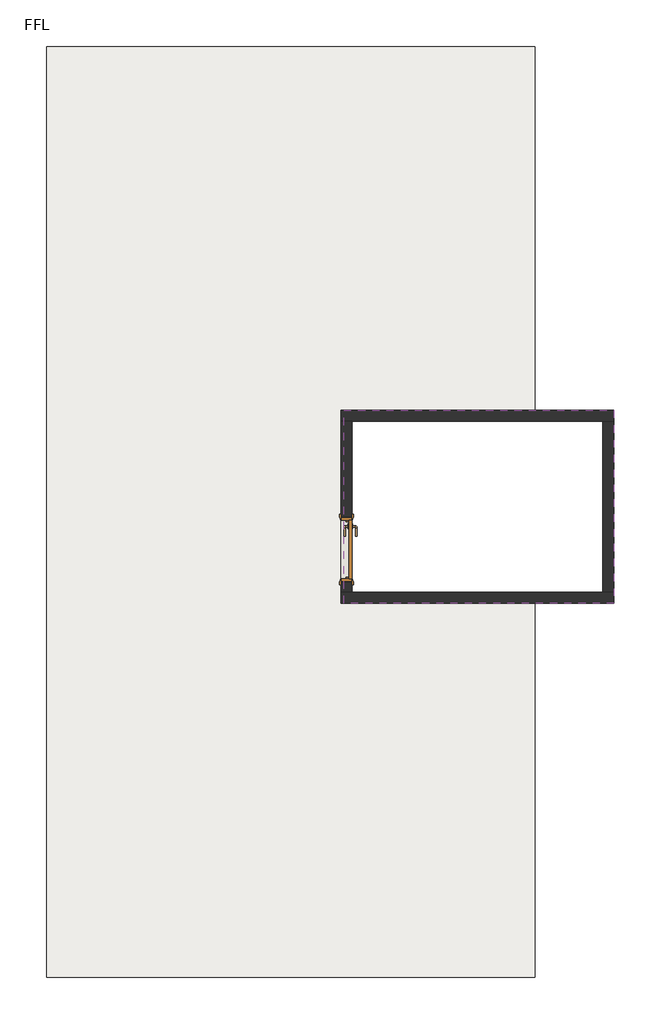
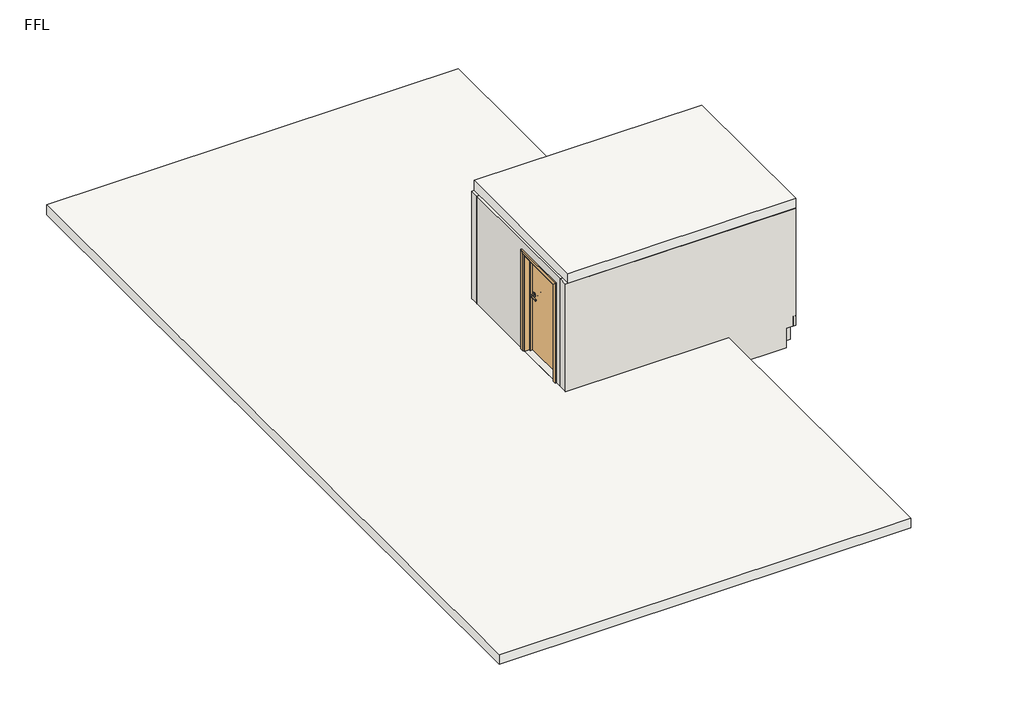
# One storey, incomplete: 4 walls, 3 slabs, 1 door.
"""IFC4 building model written with IfcOpenShell, lengths in millimetres."""

from ifc_helpers import new_model, si_unit, frame, origin, place, context, project, spatial, polyline, outline, extrude, faceted_brep, transform, mapped, element, save
from components import doors_intsgl_810x1524mm_3577b09a

model = new_model("IFC4")

# Units and contexts
model_context = context("Model", 3, world=origin())
ifc_project = project(units=[si_unit("LENGTHUNIT", "METRE", prefix="MILLI")], contexts=[model_context])

# Site, building, storey
site = spatial("IfcSite", under=ifc_project)
building = spatial("IfcBuilding", under=site)
storey = spatial("IfcBuildingStorey", under=building, Name="FFL", Elevation=3048.0)

# Door
placement = place(None, origin())
doors_intsgl_810x1524mm_shape = doors_intsgl_810x1524mm_3577b09a(model_context)
element("IfcDoor", 1, ObjectType="Doors_IntSgl : 810x1524mm", at=placement, inside=storey, context=model_context, shape_type="MappedRepresentation", body=[
    mapped(doors_intsgl_810x1524mm_shape, transform((-2390.6174044, 5851.2803577, 3200.4), x_axis=(0.0, -1.0, 0.0), y_axis=(1.0, 0.0, 0.0), z_axis=(0.0, 0.0, 1.0))),
])

# Slabs
element("IfcSlab", 2, ObjectType="SLAB", at=placement, inside=storey, context=model_context, shape_type="SweptSolid", body=[
    extrude(outline(polyline([(-42.3874044, 12109.5354997), (-42.3874044, 7583.3887671), (-2320.9121226, 7583.3887671), (-2320.9121226, 5180.7203577), (-42.3874044, 5180.7203577), (-42.3874044, 527.1354997), (-6124.4174044, 527.1354997), (-6124.4174044, 12109.5354997), (-42.3874044, 12109.5354997)])), frame((0.0, 0.0, 3048.0), z_axis=(0.0, 0.0, 1.0), x_axis=(1.0, 0.0, 0.0)), (0.0, 0.0, 1.0), 149.9616),
    extrude(outline(polyline([(941.6891182, 7583.3887671), (941.6891182, 5180.7203577), (906.3025956, 5180.7203577), (906.3025956, 7583.3887671), (941.6891182, 7583.3887671)])), frame((0.0, 0.0, 3048.0), z_axis=(0.0, 0.0, 1.0), x_axis=(1.0, 0.0, 0.0)), (0.0, 0.0, 1.0), 149.9616),
])
element("IfcSlab", 3, ObjectType="SLAB", at=placement, inside=storey, context=model_context, shape_type="SweptSolid", body=[
    extrude(outline(polyline([(941.6891182, 7583.3887671), (941.6891182, 5180.7203577), (-2421.0974044, 5180.7203577), (-2421.0974044, 7583.3887671), (941.6891182, 7583.3887671)])), frame((0.0, 0.0, 4879.2384), z_axis=(0.0, 0.0, 1.0), x_axis=(1.0, 0.0, 0.0)), (0.0, 0.0, 1.0), 149.9616),
])
element("IfcSlab", 4, ObjectType="SLAB", at=placement, inside=storey, context=model_context, shape_type="SweptSolid", body=[
    extrude(outline(polyline([(941.6891182, 7583.3887671), (941.6891182, 5180.7203577), (906.3025956, 5180.7203577), (906.3025956, 7583.3887671), (941.6891182, 7583.3887671)])), frame((0.0, 0.0, 3048.0), z_axis=(0.0, 0.0, 1.0), x_axis=(1.0, 0.0, 0.0)), (0.0, 0.0, 1.0), 149.9616),
    extrude(outline(polyline([(-2459.1974044, 5180.7203577), (-2459.1974044, 7583.3887671), (-2320.9121226, 7583.3887671), (-2320.9121226, 5180.7203577), (-2459.1974044, 5180.7203577)])), frame((0.0, 0.0, 3048.0), z_axis=(0.0, 0.0, 1.0), x_axis=(1.0, 0.0, 0.0)), (0.0, 0.0, 1.0), 149.9616),
])

# Walls
element("IfcWall", 5, ObjectType="INNER WALL", at=placement, inside=storey, context=model_context, shape_type="Brep", body=[
    faceted_brep([(-2421.0974044, 7446.2287671, 2743.2), (-2322.0374044, 7446.2287671, 2743.2), (804.5291182, 7446.2287671, 2743.2), (804.5291182, 7446.2287671, 3048.0), (941.6891182, 7446.2287671, 3048.0), (941.6891182, 7446.2287671, 4876.8), (804.5291182, 7446.2287671, 4876.8), (-2322.0374044, 7446.2287671, 4876.8), (-2459.1974044, 7446.2287671, 4876.8), (-2459.1974044, 7446.2287671, 3048.0), (-2421.0974044, 7446.2287671, 3048.0), (-2421.0974044, 7583.3887671, 2743.2), (-2421.0974044, 7583.3887671, 3048.0), (-2459.1974044, 7583.3887671, 3048.0), (-2459.1974044, 7583.3887671, 4876.8), (941.6891182, 7583.3887671, 4876.8), (941.6891182, 7583.3887671, 3048.0), (804.5291182, 7583.3887671, 3048.0), (804.5291182, 7583.3887671, 2743.2)], [[[0, 1, 2, 3, 4, 5, 6, 7, 8, 9, 10]], [[11, 12, 13, 14, 15, 16, 17, 18]], [[2, 1, 0, 11, 18]], [[8, 7, 6, 5, 15, 14]], [[16, 4, 3, 17]], [[3, 2, 18, 17]], [[5, 4, 16, 15]], [[9, 13, 12, 10]], [[0, 10, 12, 11]], [[9, 8, 14, 13]]]),
])
element("IfcWall", 6, ObjectType="INNER WALL", at=placement, inside=storey, context=model_context, shape_type="Brep", body=[
    faceted_brep([(-2459.1974044, 5180.7203577, 2743.2), (804.5291182, 5180.7203577, 2743.2), (804.5291182, 5180.7203577, 3048.0), (941.6891182, 5180.7203577, 3048.0), (941.6891182, 5180.7203577, 4876.8), (-2459.1974044, 5180.7203577, 4876.8), (-2459.1974044, 5317.8803577, 2743.2), (-2459.1974044, 5317.8803577, 4876.8), (-2322.0374044, 5317.8803577, 4876.8), (804.5291182, 5317.8803577, 4876.8), (941.6891182, 5317.8803577, 4876.8), (941.6891182, 5317.8803577, 3048.0), (804.5291182, 5317.8803577, 3048.0), (804.5291182, 5317.8803577, 2743.2), (-2322.0374044, 5317.8803577, 2743.2)], [[[0, 1, 2, 3, 4, 5]], [[6, 7, 8, 9, 10, 11, 12, 13, 14]], [[1, 0, 6, 14, 13]], [[5, 4, 10, 9, 8, 7]], [[0, 5, 7, 6]], [[11, 3, 2, 12]], [[2, 1, 13, 12]], [[4, 3, 11, 10]]]),
])
element("IfcWall", 7, ObjectType="INNER WALL", at=placement, inside=storey, context=model_context, shape_type="Brep", body=[
    faceted_brep([(941.6891182, 5317.8803577, 4876.8), (941.6891182, 5317.8803577, 3048.0), (941.6891182, 5317.8803577, 2743.2), (941.6891182, 7446.2287671, 2743.2), (941.6891182, 7446.2287671, 3048.0), (941.6891182, 7446.2287671, 4876.8), (941.6891182, 5620.0545624, 3974.1348707), (941.6891182, 7144.0545624, 3974.1348707), (941.6891182, 7144.0545624, 3064.1348707), (941.6891182, 5620.0545624, 3064.1348707), (804.5291182, 5317.8803577, 2743.2), (804.5291182, 5317.8803577, 4876.8), (804.5291182, 7446.2287671, 4876.8), (804.5291182, 7446.2287671, 2743.2), (804.5291182, 5620.0545624, 3974.1348707), (804.5291182, 5620.0545624, 3064.1348707), (804.5291182, 7144.0545624, 3064.1348707), (804.5291182, 7144.0545624, 3974.1348707)], [[[0, 1, 2, 3, 4, 5], [6, 7, 8, 9]], [[10, 11, 12, 13], [14, 15, 16, 17]], [[3, 2, 10, 13]], [[0, 5, 12, 11]], [[0, 11, 10, 2, 1]], [[3, 13, 12, 5, 4]], [[15, 14, 6, 9]], [[16, 15, 9, 8]], [[17, 16, 8, 7]], [[14, 17, 7, 6]]]),
])
element("IfcWall", 8, ObjectType="INNER WALL", at=placement, inside=storey, context=model_context, shape_type="Brep", body=[
    faceted_brep([(-2459.1974044, 7446.2287671, 2743.2), (-2459.1974044, 5317.8803577, 2743.2), (-2459.1974044, 5317.8803577, 4876.8), (-2459.1974044, 7446.2287671, 4876.8), (-2459.1974044, 7446.2287671, 3048.0), (-2459.1974044, 5446.2803577, 4724.4), (-2459.1974044, 5446.2803577, 3200.4), (-2459.1974044, 6256.2803577, 3200.4), (-2459.1974044, 6256.2803577, 4724.4), (-2322.0374044, 5317.8803577, 2743.2), (-2322.0374044, 7446.2287671, 2743.2), (-2322.0374044, 7446.2287671, 4876.8), (-2322.0374044, 5317.8803577, 4876.8), (-2322.0374044, 5446.2803577, 3200.4), (-2322.0374044, 5446.2803577, 4724.4), (-2322.0374044, 6256.2803577, 4724.4), (-2322.0374044, 6256.2803577, 3200.4), (-2421.0974044, 7446.2287671, 2743.2)], [[[0, 1, 2, 3, 4], [5, 6, 7, 8]], [[9, 10, 11, 12], [13, 14, 15, 16]], [[1, 0, 17, 10, 9]], [[3, 2, 12, 11]], [[13, 6, 5, 14]], [[14, 5, 8, 15]], [[15, 8, 7, 16]], [[6, 13, 16, 7]], [[1, 9, 12, 2]], [[10, 17, 0, 4, 3, 11]]]),
])

save(model, "model.ifc")

# Revit data of these elements
# Type "Doors_IntSgl : 810x1524mm"
#   Construction Type Id = "MDOOR"
#   Type Mark = "42"
#   Type Comments = "Internal Single"
#   Operation = "SingleSwingRight"
#   Manufacturer = "Revit"
#   Keynote = "L20"
#   Description = "Internal Single Door"
#   Analytic Construction = "Metal"
#   UnderCut = 8 mm
#   Tolerance = 2 mm
#   Thickness = 38 mm
#   Thermal Resistance (R) = 0.270117 (m²·K)/W
#   Structural Tolerance = 8 mm
#   StopDepth = 32 mm
#   Stop Thickness = 19 mm
#   Rough Width = 810 mm
#   Rough Height = 1524 mm
#   Height to Top Lock Rail = 1000 mm
#   Heat Transfer Coefficient (U) = 3.7021 W/(m²·K)
#   Handle Z Distance = 900 mm
#   Handle X Distance = 75 mm
#   Frame Thickness = 32 mm
#   Door Panel Width = 726 mm
#   Door Panel Thickness = 38 mm
#   Door Panel Offset = 0 mm
#   Height = 1524 mm
#   Width = 810 mm
#   Door Panel Height = 1474 mm
#   Architrave Setback = 5 mm
#   Define Thermal Properties by = 1
#   Vis - Ironmongery = yes
#   Material Ironmongery = Door - Handle
#   Material Frame = Door - Frame/Mullion (1)
#   Material Door = Door - Panel
#   Material Architrave = Door - Architrave
#   Visual Light Transmittance = 0
#   Solar Heat Gain Coefficient = 0
#   Function = (empty or 0)
#   Wall Closure = (empty or 0)
# Type "SLAB"
#   Layers, outside or top first: 149.962 mm "Concrete, Cast In Situ" (function 1)
# Type "INNER WALL"
#   Keynote = "F10"
#   Layers, outside or top first: 137.16 mm "Brick, Common" (function 1)
# Element 1 (IfcDoor, "Doors_IntSgl : 810x1524mm")
#   Phase Created = New Construction
#   Materials on its faces: "Door - Architrave", "Door - Handle", "Door - Frame/Mullion (1)", "Door - Panel"
# Elements 2, 4 (IfcSlab, "SLAB")
#   Height Offset From Level = 149.962 mm
#   built-in parameter 1001954 = 1
#   Phase Created = New Construction
#   Materials on its faces: "Concrete, Cast In Situ"
# Element 3 (IfcSlab, "SLAB")
#   Height Offset From Level = 1981.2 mm
#   built-in parameter 1001954 = 1
#   Phase Created = New Construction
#   Materials on its faces: "Concrete, Cast In Situ"
# Elements 5, 6, 7, 8 (IfcWall, "INNER WALL")
#   built-in parameter 1001111 = -304.8 mm
#   Top Offset = 0 mm
#   Base Offset = -304.8 mm
#   Unconnected Height = 2133.6 mm
#   wall height = 2133.6 mm
#   Phase Created = New Construction
#   Base Constraint = FFL
#   Materials on its faces: "Brick, Common"
# Materials
#   "Door - Handle": colour RGB 0 0 0, transparency 0, Keynote = "P21", Cost = 0
#   "Door - Frame/Mullion (1)": class "Wood", colour RGB 212 179 113, transparency 0, Keynote = "L20", Cost = 0
#   "Door - Panel": class "Wood", colour RGB 210 159 95, transparency 0, Keynote = "L20", Cost = 0
#   "Door - Architrave": class "Wood", colour RGB 154 90 5, transparency 0, Keynote = "P20", Cost = 0
#   "Concrete, Cast In Situ": class "Concrete", colour RGB 192 192 192, transparency 0, Description = "physical material", Cost = 0
#   "Brick, Common": class "Masonry", colour RGB 170 100 105, transparency 0, Description = "Common brick", Cost = 0
